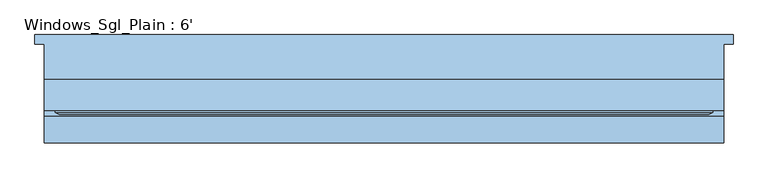
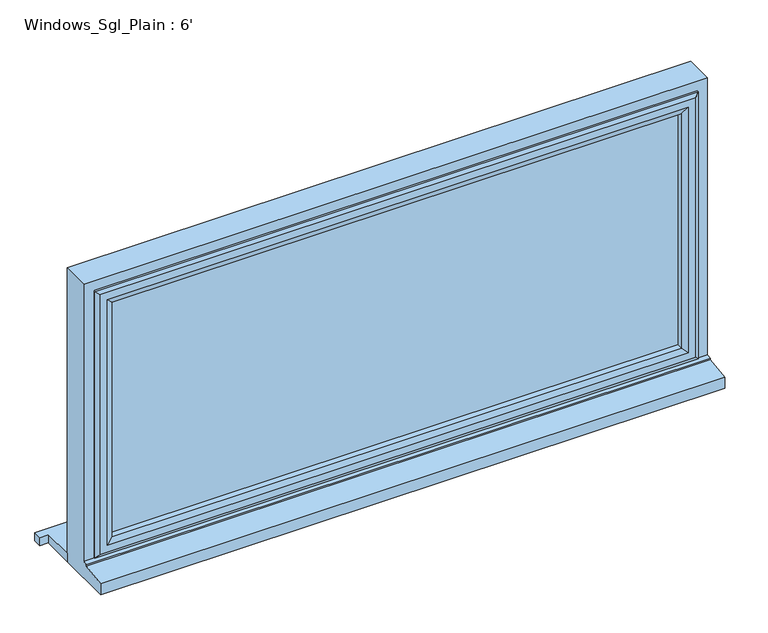
"""IFC4 building model written with IfcOpenShell, lengths in millimetres: window geometry, Windows_Sgl_Plain : 6'."""

from ifc_helpers import new_model, si_unit, frame, origin, place, context, project, spatial, polyline, outline, extrude, faceted_brep, source, transform, mapped, element, save


def windows_sgl_plain_6_3dcb7f7b(model_context):
    return source(origin(), model_context, "Body", "SolidModel", [
        extrude(outline(polyline([(-939.4, 130.8434322), (939.4, 130.8434322), (939.4, 105.8434322), (914.4, 105.8434322), (914.4, 10.2434322), (-914.4, 10.2434322), (-914.4, 105.8434322), (-939.4, 105.8434322), (-939.4, 130.8434322)])), frame((0.0, 0.0, 1200.0), z_axis=(0.0, 0.0, 1.0), x_axis=(1.0, 0.0, 0.0)), (0.0, 0.0, 1.0), 25.0),
        faceted_brep([(-914.4, 10.2434322, 1200.0), (-914.4, 10.2434322, 2110.0), (914.4, 10.2434322, 2110.0), (914.4, 10.2434322, 1200.0), (-854.4, 10.2434322, 2050.0), (-854.4, 10.2434322, 1275.0), (854.4, 10.2434322, 1275.0), (854.4, 10.2434322, 2050.0), (-914.4, -160.2565678, 1200.0), (-914.4, -160.2565678, 1233.8088847), (-914.4, -87.7565678, 1244.7449676), (-914.4, -87.7565678, 1249.68767), (-914.4, -72.7565678, 1251.0), (-914.4, -72.7565678, 2110.0), (914.4, -72.7565678, 1251.0), (914.4, -72.7565678, 2110.0), (-874.4, -72.7565678, 2070.0), (874.4, -72.7565678, 2070.0), (874.4, -72.7565678, 1263.0), (-874.4, -72.7565678, 1263.0), (-874.4, -7.7565678, 1263.0), (-874.4, -7.7565678, 2070.0), (874.4, -7.7565678, 1263.0), (874.4, -7.7565678, 2070.0), (-854.4, -7.7565678, 2050.0), (854.4, -7.7565678, 2050.0), (854.4, -7.7565678, 1275.0), (-854.4, -7.7565678, 1275.0), (914.4, -87.7565678, 1249.68767), (914.4, -87.7565678, 1244.7449676), (914.4, -160.2565678, 1233.8088847), (914.4, -160.2565678, 1200.0)], [[[0, 1, 2, 3], [4, 5, 6, 7]], [[0, 8, 9, 10, 11, 12, 13, 1]], [[12, 14, 15, 13], [16, 17, 18, 19]], [[19, 20, 21, 16]], [[21, 20, 22, 23], [24, 25, 26, 27]], [[24, 27, 5, 4]], [[1, 13, 15, 2]], [[16, 21, 23, 17]], [[7, 25, 24, 4]], [[14, 28, 29, 30, 31, 3, 2, 15]], [[17, 23, 22, 18]], [[7, 6, 26, 25]], [[31, 8, 0, 3]], [[30, 9, 8, 31]], [[29, 10, 9, 30]], [[28, 11, 10, 29]], [[14, 12, 11, 28]], [[20, 19, 18, 22]], [[5, 27, 26, 6]]]),
        extrude(outline(polyline([(844.4, -36.7565678), (844.4, -60.7565678), (-844.4, -60.7565678), (-844.4, -36.7565678), (844.4, -36.7565678)])), frame((0.0, 0.0, 1293.0), z_axis=(0.0, 0.0, 1.0), x_axis=(1.0, 0.0, 0.0)), (0.0, 0.0, 1.0), 747.0),
        faceted_brep([(-884.4, -72.7565678, 2080.0), (-884.4, -72.7565678, 1253.0), (-884.4, -78.5300705, 1253.0), (-884.4, -78.5300705, 2080.0), (-874.4, -7.7565678, 2070.0), (-874.4, -7.7565678, 1263.0), (-874.4, -72.7565678, 1263.0), (-874.4, -72.7565678, 2070.0), (-834.4, -22.2494677, 2030.0), (-834.4, -22.2494677, 1303.0), (-844.5480377, -7.7565678, 1292.8519623), (-844.5480377, -7.7565678, 2040.1480377), (-834.4, -36.7565678, 2030.0), (-834.4, -36.7565678, 1303.0), (-844.4, -60.7565678, 2040.0), (-844.4, -60.7565678, 1293.0), (-844.4, -36.7565678, 1293.0), (-844.4, -36.7565678, 2040.0), (-834.4, -78.5300705, 2030.0), (-834.4, -78.5300705, 1303.0), (-834.4, -60.7565678, 1303.0), (-834.4, -60.7565678, 2030.0), (-851.8457548, -84.3035732, 2047.4457548), (-851.8457548, -84.3035732, 1285.5542452), (-873.6153903, -84.3035732, 1263.7846097), (-873.6153903, -84.3035732, 2069.2153903), (884.4, -72.7565678, 1253.0), (884.4, -78.5300705, 1253.0), (874.4, -7.7565678, 1263.0), (874.4, -72.7565678, 1263.0), (834.4, -22.2494677, 1303.0), (844.5480377, -7.7565678, 1292.8519623), (834.4, -36.7565678, 1303.0), (844.4, -60.7565678, 1293.0), (844.4, -36.7565678, 1293.0), (834.4, -78.5300705, 1303.0), (834.4, -60.7565678, 1303.0), (851.8457548, -84.3035732, 1285.5542452), (873.6153903, -84.3035732, 1263.7846097), (884.4, -72.7565678, 2080.0), (884.4, -78.5300705, 2080.0), (874.4, -7.7565678, 2070.0), (874.4, -72.7565678, 2070.0), (834.4, -22.2494677, 2030.0), (844.5480377, -7.7565678, 2040.1480377), (834.4, -36.7565678, 2030.0), (844.4, -60.7565678, 2040.0), (844.4, -36.7565678, 2040.0), (834.4, -78.5300705, 2030.0), (834.4, -60.7565678, 2030.0), (851.8457548, -84.3035732, 2047.4457548), (873.6153903, -84.3035732, 2069.2153903)], [[[0, 1, 2, 3]], [[4, 5, 6, 7]], [[8, 9, 10, 11]], [[12, 13, 9, 8]], [[14, 15, 16, 17]], [[18, 19, 20, 21]], [[22, 23, 19, 18]], [[3, 2, 24, 25]], [[1, 26, 27, 2]], [[5, 28, 29, 6]], [[9, 30, 31, 10]], [[13, 32, 30, 9]], [[15, 33, 34, 16]], [[19, 35, 36, 20]], [[23, 37, 35, 19]], [[2, 27, 38, 24]], [[26, 39, 40, 27]], [[28, 41, 42, 29]], [[30, 43, 44, 31]], [[32, 45, 43, 30]], [[33, 46, 47, 34]], [[35, 48, 49, 36]], [[37, 50, 48, 35]], [[27, 40, 51, 38]], [[39, 0, 3, 40]], [[1, 0, 39, 26], [7, 6, 29, 42]], [[41, 4, 7, 42]], [[5, 4, 41, 28], [11, 10, 31, 44]], [[43, 8, 11, 44]], [[45, 12, 8, 43]], [[17, 16, 34, 47], [13, 12, 45, 32]], [[46, 14, 17, 47]], [[15, 14, 46, 33], [21, 20, 36, 49]], [[48, 18, 21, 49]], [[50, 22, 18, 48]], [[25, 24, 38, 51], [23, 22, 50, 37]], [[40, 3, 25, 51]]]),
    ])


if __name__ == "__main__":
    model = new_model("IFC4")
    model_context = context("Model", 3, world=origin())
    ifc_project = project(units=[si_unit("LENGTHUNIT", "METRE", prefix="MILLI")], contexts=[model_context])
    site = spatial("IfcSite", under=ifc_project)
    building = spatial("IfcBuilding", under=site)
    placement = place(None, origin())
    windows_sgl_plain_6_shape = windows_sgl_plain_6_3dcb7f7b(model_context)
    element("IfcWindow", 1, ObjectType="Windows_Sgl_Plain : 6'", at=placement, inside=building, context=model_context, shape_type="MappedRepresentation", body=[
        mapped(windows_sgl_plain_6_shape, transform((0.0, 0.0, 0.0), x_axis=(1.0, 0.0, 0.0), y_axis=(0.0, 1.0, 0.0), z_axis=(0.0, 0.0, 1.0))),
    ])
    save(model, "model.ifc")

# Revit data of these elements
# Type "Windows_Sgl_Plain : 6'"
#   Type Mark = "69"
#   Operation = "SinglePanel"
#   Construction Type Id = "SGL"
#   Manufacturer = "Revit"
#   Keynote = "L10"
#   Analytic Construction = "Large single-glazed windows"
#   Wrap Layers (Ext) from Ext = 0' - 4.03543"
#   Wrap Layers (Int) from Ext = 0' - 6.98819"
#   Window Board Projection = 0' - 0.98425"
#   Window Board Extension = 0' - 0.98425"
#   Visual Light Transmittance = 0.9
#   Solar Heat Gain Coefficient = 0.86
#   Rough Width = 6' - 0"
#   Rough Height = 2' - 11.82677"
#   Height = 2' - 11.82677"
#   Width = 6' - 0"
#   Heat Transfer Coefficient (U) = 5.5617 W/(m²·K)
#   Glazing Thickness = 0' - 0.94488"
#   FrameOffset - External = 0' - 1.9685"
#   Frame Depth = 0' - 2.55906"
#   Default Head Height = 6' - 11.07087"
#   Cill Depth = 0' - 3.44488"
#   Cavity Closer Width = 0' - 1.9685"
#   Cavity Closer Offset from Ext = 0' - 4.03543"
#   Cavity Closer Depth = 0' - 3.34646"
#   Vis - Cavity Closers = yes
#   Define Thermal Properties by = 1
#   Material Trim = Window Frame
#   Material Glass = Glass
#   Material Frame = Window Frame
#   Wall Closure = (empty or 0)
# Element 1 (IfcWindow, "Windows_Sgl_Plain : 6'")
#   Materials on its faces: "Window Frame", "Glass"
# Materials
#   "Window Frame": colour RGB 249 249 249, transparency 0, Keynote = "L10", Cost = 0
#   "Glass": class "Glass", colour RGB 0 128 192, transparency 0.9, Description = "Soda Lime Glass", Cost = 0
